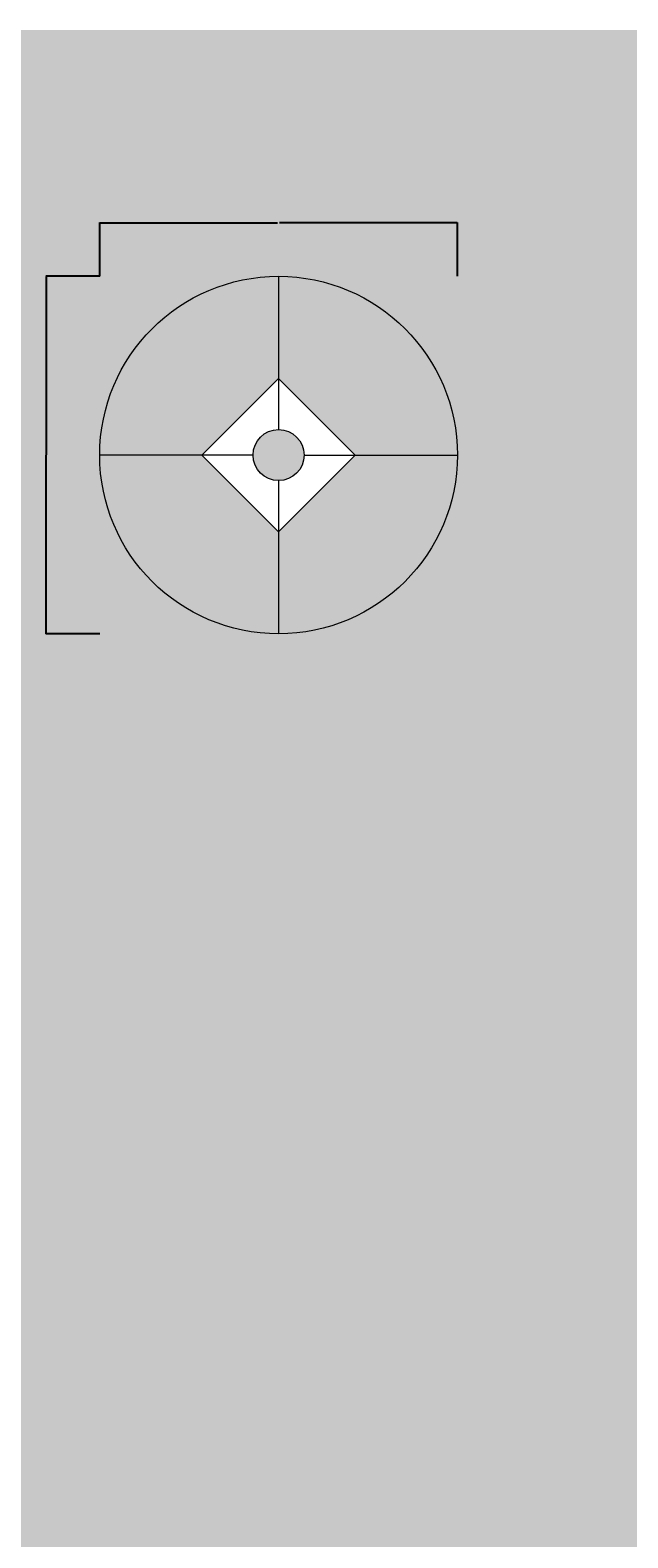
# Model space of a CAD drawing. Units: millimetres. Extents: x -229 to 16545, y -10488 to 4272.
# Tile 19 of 29: x 10978 to 11572, y -2708 to -1208. Entities that reach past the tile are written whole.
import ezdxf

# ---------------------------------------------------------------- set-up
doc = ezdxf.new("R2010")
doc.units = ezdxf.units.MM
for name, color, linetype, lineweight in [('A-ANNO-DIMS', 2, 'Continuous', 18), ('A-FURN', 8, 'Continuous', 18), ('A-FURN-PATT', 252, 'Continuous', 13)]:
    doc.layers.add(name, color=color, linetype=linetype, lineweight=lineweight)
doc.layers.add('A-FLOR-PATT', color=254, linetype='Continuous', lineweight=13, true_color=0xfeeab9)
doc.styles.get("Standard").update_dxf_attribs({"font": 'arial.ttf'})
doc.dimstyles.get("Standard").update_dxf_attribs({"dimtxt": 0.18, "dimasz": 0.18, "dimexe": 0.18, "dimexo": 0.0625, "dimgap": 0.09, "dimtad": 0, "dimtih": 1, "dimtoh": 1, "dimdec": 4, "dimzin": 0, "dimdsep": 46, "dimtxsty": 'Standard', "dimcen": 0.09, "dimadec": 0, "dimazin": 0, "dimtfac": 1, "dimtdec": 4, "dimtofl": 0, "dimtmove": 0, "dimatfit": 3, "dimfxl": 1, "dimtolj": 1, "dimtzin": 0, "dimarcsym": 0})

# ---------------------------------------------------------------- blocks, each defined once
blk = doc.blocks.new('Lamp - Table')
for p, q in [((0, 7), (0, 1)), ((0, 3), (-3, 0)), ((3, 0), (0, 3)), ((-1, 0), (-7, 0)), ((-3, 0), (0, -3)), ((0, -3), (3, 0)), ((1, 0), (7, 0)), ((0, -1), (0, -7))]:
    blk.add_line(p, q)
for radius in [7, 1]:
    blk.add_circle((0, 0), radius)
blk = doc.blocks.new('*D27')
at = {"layer": 'A-ANNO-DIMS', "color": 0, "lineweight": -2, "transparency": 16777216}
for p, q in [((11047.2, -1453.1), (11047.2, -1399.6)), ((11047.4, -1399.8), (11224, -1399.8)), ((11402.6, -1399.8), (11226, -1399.8)), ((11402.8, -1453.1), (11402.8, -1399.6))]:
    blk.add_line(p, q, dxfattribs=at)
at = {"layer": 'A-ANNO-DIMS', "color": 0, "transparency": 16777216}
for points in [[(11047.4, -1399.8), (11047.4, -1399.8), (11047.2, -1399.8)], [(11402.6, -1399.8), (11402.6, -1399.8), (11402.8, -1399.8)]]:
    blk.add_solid(points, dxfattribs=at)
at = {"layer": 'Defpoints', "color": 0, "transparency": 16777216}
for p in [(11402.8, -1399.8), (11047.2, -1453.1), (11402.8, -1453.1)]:
    blk.add_point(p, dxfattribs=at)
at = {"layer": 'A-ANNO-DIMS', "color": 0, "transparency": 16777216, "insert": (11225, -1399.8), "char_height": 0.18, "attachment_point": 5}
blk.add_mtext('\\A1;LAMP 356 TYP.', dxfattribs=at)
blk = doc.blocks.new('*D28')
at = {"layer": 'A-ANNO-DIMS', "color": 0, "lineweight": -2, "transparency": 16777216}
for p, q in [((11047.2, -1453.1), (10993.7, -1453.1)), ((10993.9, -1453.3), (10993.9, -1630.8)), ((10993.9, -1808.6), (10993.9, -1631.1)), ((11047.2, -1808.7), (10993.7, -1808.7))]:
    blk.add_line(p, q, dxfattribs=at)
at = {"layer": 'A-ANNO-DIMS', "color": 0, "transparency": 16777216}
for points in [[(10993.8, -1453.3), (10993.9, -1453.3), (10993.9, -1453.1)], [(10993.8, -1808.6), (10993.9, -1808.6), (10993.9, -1808.7)]]:
    blk.add_solid(points, dxfattribs=at)
at = {"layer": 'Defpoints', "color": 0, "transparency": 16777216}
for p in [(10993.9, -1453.1), (11047.2, -1453.1), (11047.2, -1808.7)]:
    blk.add_point(p, dxfattribs=at)
at = {"layer": 'A-ANNO-DIMS', "color": 0, "transparency": 16777216, "insert": (10993.9, -1630.9), "char_height": 0.18, "attachment_point": 5}
blk.add_mtext('\\A1;356 TYP.', dxfattribs=at)

msp = doc.modelspace()

# ---------------------------------------------------------------- hatches: boundary and pattern name
at = {"layer": 'A-FLOR-PATT', "transparency": 33554592}
h = msp.add_hatch(color=256, dxfattribs=at)
h.dxf.hatch_style = 1
h.paths.add_polyline_path([(7975.933, -5325.772), (7943.121, -5325.772), (7943.121, -4576.49, 0.40145271), (7225.933, -5325.772, 0.40145271), (6508.746, -4576.49), (6508.746, -5325.772), (6475.933, -5325.772), (6475.933, -5438.272), (5975.933, -5438.272), (5975.933, -7267.724), (5975.933, -7438.272), (6478.619, -7438.272), (6463.448, -7355.919), (6464.88, -7356.837), (6463.849, -7358.097), (6478.619, -7438.272), (6610.327, -7438.272), (6632.656, -7409.564), (6632.525, -7406.967), (6634.208, -7407.569), (6619.273, -7426.77), (6654.466, -7438.272), (7610.517, -7438.272), (7607.41, -7421.409), (7608.842, -7422.327), (7607.812, -7423.587), (7610.517, -7438.272), (7975.933, -7438.272)])
h.paths.add_polyline_path([(13785.933, -1208.272), (9555.933, -1208.272), (9555.933, -961.785), (9705.933, -961.785), (9705.933, -918.035), (10704.976, -918.035, 0.40145271), (9705.933, 38.215), (9555.933, 38.215), (9555.933, 2021.728), (5975.933, 2021.728), (5975.933, 755.492), (5745.933, 755.492), (5745.933, 1427.266), (2918.813, 1427.266), (2918.813, -492.942), (5013.319, -492.942), (5013.319, -978.272), (5745.933, -978.272), (5745.933, -397.513), (5975.933, -397.513), (5975.933, -1208.272), (4560.933, -1208.272), (4560.933, -1265.772), (4448.433, -1265.772), (4448.433, -1298.585), (4445.933, -1298.585), (3699.151, -1298.585, 0.40145271), (4448.433, -2015.772), (4560.933, -2015.772), (4560.933, -2384.177), (5745.933, -2384.177), (5799.402, -2384.177), (5799.402, -4518.272), (5975.933, -4518.272), (5975.933, -5208.272), (6475.933, -5208.272), (6475.933, -4575.772), (6508.746, -4575.772), (6508.746, -4576.49, -0.35647263), (7216.672, -5208.272), (7235.194, -5208.272, -0.35647263), (7943.121, -4576.49), (7943.121, -4575.772), (7975.933, -4575.772), (7975.933, -5208.272), (11176.247, -5208.272), (11159.44, -5191.465), (10520.768, -5191.465), (10520.768, -4888.936), (10571.19, -4888.936), (10571.19, -4872.129), (10772.876, -4872.129), (10772.876, -4888.936), (10789.683, -4888.936), (10789.683, -4872.129), (10991.368, -4872.129), (10991.368, -4888.936), (11041.79, -4888.936), (11041.79, -4872.129), (11058.597, -4872.129, -0.09090909), (11428.354, -4872.129), (11445.162, -4872.129), (11445.162, -4888.936), (11529.197, -4888.936), (11529.197, -5191.465), (11327.512, -5191.465), (11310.704, -5208.272), (13785.933, -5208.272)])
h.paths.add_polyline_path([(11047.216, -1630.944, -1), (11402.816, -1630.944, -1)], flags=16)
h.paths.add_polyline_path([(11148.816, -1630.944), (11225.016, -1554.744), (11301.216, -1630.944), (11225.016, -1707.144)], flags=0)
h.paths.add_polyline_path([(11199.616, -1630.944, -1), (11250.416, -1630.944, -1)], flags=0)
h.paths.add_polyline_path([(11588.751, -2096.259), (11588.751, -1543.254, -0.26666697), (12864.918, -1543.254), (12864.918, -2096.259), (12737.302, -2096.259), (12737.302, -2063.121), (11716.368, -2063.121), (11716.368, -2096.259)], flags=16)
h.paths.add_polyline_path([(12012.696, -2489.42), (12600.997, -2489.42), (12600.997, -3666.022), (12012.696, -3666.022)], flags=16)
h.paths.add_polyline_path([(12176.41, -3599.403), (12174.938, -3609.076), (12173.789, -3618.819), (12173.09, -3628.559), (12172.973, -3638.221), (12173.89, -3652.852), (12175.008, -3657.025), (12172.909, -3643.473), (12173.142, -3624.297), (12175.386, -3605.273)], flags=0)
h.paths.add_polyline_path([(8026.289, -286.944), (7737.703, -287.19), (7734.87, -269.156), (8029.092, -268.905)], flags=16)
h.paths.add_polyline_path([(7733.453, -260.139), (7710.784, -115.865), (7557.191, -115.996), (7556.999, 109.744), (7412.687, 132.166), (7412.433, 429.206), (7556.707, 451.876), (7556.568, 614.769), (7412.256, 637.19), (7412.003, 934.231), (7556.276, 956.9), (7556.084, 1182.639), (7709.677, 1182.77), (7732.099, 1327.082), (8029.14, 1327.335), (8051.808, 1183.062), (8205.401, 1183.192), (8205.594, 957.454), (8349.906, 935.031), (8350.159, 637.99), (8205.885, 615.322), (8206.024, 452.43), (8350.336, 430.006), (8350.59, 132.965), (8206.316, 110.298), (8206.509, -115.442), (8052.916, -115.573), (8030.493, -259.885)], flags=16)
h.paths.add_polyline_path([(12261.416, -3475.554), (12262.632, -3486.776), (12264.032, -3497.007), (12265.554, -3506.365), (12267.136, -3514.968), (12268.719, -3522.935), (12271.304, -3535.59), (12273.606, -3548.078), (12275.271, -3561.064), (12275.93, -3574.938), (12275.325, -3590.3), (12273.425, -3607.964), (12270.795, -3625.658), (12268.066, -3641.063), (12266.318, -3649.679), (12265.456, -3653.626), (12263.984, -3659.846), (12264.032, -3659.566), (12264.342, -3658.241), (12264.807, -3656.37), (12265.456, -3653.626), (12266.318, -3649.679), (12267.409, -3644.302), (12268.668, -3637.664), (12270.019, -3630.037), (12271.384, -3621.695), (12272.69, -3612.908), (12273.857, -3603.948), (12274.81, -3595.088), (12275.47, -3586.601), (12275.782, -3578.689), (12275.757, -3571.292), (12275.423, -3564.275), (12274.816, -3557.512), (12273.964, -3550.872), (12272.896, -3544.224), (12271.645, -3537.439), (12270.24, -3530.385), (12267.543, -3517.181), (12264.612, -3501.247), (12261.849, -3481.059)], flags=0)
h.paths.add_polyline_path([(12332.136, -3408.03), (12333.483, -3416.79), (12335.077, -3424.54), (12336.915, -3431.355), (12338.991, -3437.32), (12341.266, -3442.55), (12343.694, -3447.166), (12346.229, -3451.292), (12348.826, -3455.051), (12351.438, -3458.563), (12357.476, -3466.491), (12363.61, -3476.575), (12368.309, -3489.762), (12369.929, -3503.427), (12369.842, -3516.511), (12368.43, -3530.867), (12365.816, -3545.835), (12362.382, -3559.786), (12360.968, -3564.487), (12363.063, -3557.021), (12364.898, -3549.566), (12366.473, -3542.077), (12367.773, -3534.631), (12368.781, -3527.301), (12369.483, -3520.162), (12369.863, -3513.291), (12369.906, -3506.759), (12369.599, -3500.643), (12368.93, -3494.999), (12367.924, -3489.796), (12366.61, -3484.994), (12365.024, -3480.542), (12363.19, -3476.399), (12361.141, -3472.516), (12358.909, -3468.847), (12356.525, -3465.347), (12354.02, -3461.954), (12351.438, -3458.563), (12345.462, -3450.529), (12339.923, -3439.996), (12335.85, -3428.296), (12332.68, -3412.888)], flags=0)
h.paths.add_polyline_path([(12385.287, -3334.612), (12384.977, -3342.409), (12385.02, -3349.196), (12385.4, -3355.066), (12386.104, -3360.105), (12387.112, -3364.41), (12388.412, -3368.071), (12389.987, -3371.181), (12391.823, -3373.832), (12393.919, -3376.097), (12396.337, -3377.978), (12399.153, -3379.462), (12402.445, -3380.531), (12406.289, -3381.172), (12410.758, -3381.371), (12415.935, -3381.106), (12421.893, -3380.368), (12428.658, -3379.159), (12436.069, -3377.55), (12443.907, -3375.635), (12451.961, -3373.505), (12460.015, -3371.254), (12467.853, -3368.971), (12475.263, -3366.749), (12482.029, -3364.68), (12491.877, -3361.657), (12497.701, -3360.107), (12501.639, -3359.288), (12510.135, -3358.326), (12519.662, -3365.412), (12524.243, -3378.911), (12523.764, -3390.7), (12520.746, -3401.577), (12514.248, -3415.634), (12511.518, -3420.418), (12515.856, -3412.154), (12519.153, -3405.024), (12521.516, -3398.804), (12523.049, -3393.276), (12523.865, -3388.212), (12524.059, -3383.441), (12523.7, -3378.958), (12522.853, -3374.815), (12521.576, -3371.054), (12519.931, -3367.722), (12517.982, -3364.865), (12515.786, -3362.529), (12513.405, -3360.758), (12510.877, -3359.588), (12508.136, -3358.982), (12505.086, -3358.897), (12501.639, -3359.288), (12497.701, -3360.107), (12493.183, -3361.309), (12487.988, -3362.851), (12476.403, -3366.408), (12463.335, -3370.326), (12447.372, -3374.788), (12431.759, -3378.604), (12418.504, -3380.974), (12405.811, -3381.624), (12394.725, -3378.025), (12388.039, -3368.367), (12385.583, -3357.877), (12384.826, -3346.204), (12385.428, -3331.059), (12385.953, -3325.719)], flags=0)
h.paths.add_polyline_path([(7880.016, 1173.969), (7880.373, 1175.495), (7880.433, 1175.851), (7879.484, 1171.818)], flags=0)
h.paths.add_polyline_path([(7802.33, 874.962), (7800.771, 885.032), (7798.932, 893.941), (7796.811, 901.774), (7794.419, 908.63), (7791.798, 914.639), (7789.002, 919.945), (7786.083, 924.686), (7783.093, 929.005), (7780.087, 933.043), (7774.996, 939.717), (7768.406, 949.37), (7762.174, 963.427), (7759.342, 978.002), (7758.629, 991.888), (7759.492, 1007.928), (7761.801, 1025.496), (7765.392, 1044.035), (7766.625, 1049.048), (7764.522, 1039.543), (7762.719, 1030.232), (7761.232, 1021.168), (7760.08, 1012.405), (7759.28, 1003.994), (7758.849, 995.988), (7758.806, 988.44), (7759.167, 981.404), (7759.942, 974.914), (7761.104, 968.936), (7762.617, 963.414), (7764.448, 958.299), (7766.559, 953.535), (7768.918, 949.073), (7771.487, 944.856), (7774.232, 940.835), (7777.115, 936.938), (7782.377, 930.041), (7787.845, 922.139), (7793.348, 911.698), (7798.042, 898.247), (7801.702, 880.527)], flags=0)
h.paths.add_polyline_path([(12519.068, -3228.534), (12519.615, -3236.235), (12520.529, -3242.343), (12521.78, -3247.103), (12523.337, -3250.758), (12525.171, -3253.556), (12527.248, -3255.709), (12529.522, -3257.296), (12531.95, -3258.361), (12534.486, -3258.949), (12537.082, -3259.11), (12539.694, -3258.888), (12542.277, -3258.329), (12544.781, -3257.478), (12547.173, -3256.388), (12549.46, -3255.129), (12550.455, -3254.517), (12555.825, -3251.109), (12557.835, -3249.942), (12565.181, -3246.404), (12574.565, -3253.032), (12576.931, -3265.022), (12576.627, -3277.425), (12575.416, -3290.819), (12574.851, -3295.392), (12575.708, -3287.593), (12576.322, -3280.806), (12576.688, -3274.939), (12576.812, -3269.899), (12576.688, -3265.593), (12576.322, -3261.932), (12575.708, -3258.822), (12574.851, -3256.172), (12573.753, -3253.905), (12572.439, -3252.005), (12570.943, -3250.474), (12569.293, -3249.309), (12567.523, -3248.513), (12565.658, -3248.083), (12563.732, -3248.022), (12561.777, -3248.328), (12559.814, -3248.989), (12557.835, -3249.942), (12555.825, -3251.109), (12553.77, -3252.413), (12551.652, -3253.78), (12549.46, -3255.129), (12543.167, -3258.594), (12532.661, -3259.485), (12524.685, -3253.923), (12520.949, -3245.152), (12519.138, -3233.042)], flags=0)
h.paths.add_polyline_path([(7741.293, 790.501), (7741.641, 799.467), (7741.584, 807.269), (7741.141, 814.015), (7740.329, 819.809), (7739.165, 824.757), (7737.667, 828.966), (7735.853, 832.541), (7733.74, 835.586), (7731.348, 838.188), (7728.71, 840.348), (7725.861, 842.052), (7722.836, 843.28), (7719.671, 844.015), (7716.4, 844.237), (7713.06, 843.932), (7709.684, 843.081), (7706.304, 841.686), (7702.923, 839.834), (7699.543, 837.629), (7696.164, 835.178), (7692.784, 832.585), (7684.718, 826.315), (7675.609, 820.63), (7664.001, 817.274), (7654.105, 821.884), (7647.171, 832.02), (7644.191, 846.522), (7646.321, 860.288), (7647.49, 864.223), (7645.946, 857.865), (7645.046, 852.044), (7644.827, 846.557), (7645.243, 841.404), (7646.221, 836.642), (7647.693, 832.318), (7649.587, 828.489), (7651.832, 825.206), (7654.359, 822.523), (7657.097, 820.49), (7659.984, 819.145), (7662.993, 818.452), (7666.108, 818.357), (7669.311, 818.809), (7672.583, 819.755), (7675.908, 821.139), (7679.268, 822.913), (7682.645, 825.021), (7686.025, 827.401), (7689.404, 829.958), (7692.784, 832.585), (7700.505, 838.509), (7709.871, 843.64), (7721.436, 844.698), (7733.277, 837.617), (7739.571, 825.214), (7741.557, 811.049), (7741.669, 795.575)], flags=0)
h.paths.add_polyline_path([(8377.641, 137.216), (8359.607, 134.382), (8359.356, 428.605), (8377.395, 425.802)], flags=16)
h.paths.add_polyline_path([(7650.715, 668.465), (7650.08, 677.319), (7649.023, 684.34), (7647.579, 689.811), (7645.785, 694.012), (7643.675, 697.228), (7641.286, 699.7), (7638.669, 701.521), (7635.876, 702.744), (7632.96, 703.419), (7629.974, 703.601), (7626.971, 703.344), (7624.004, 702.697), (7621.125, 701.717), (7618.375, 700.462), (7615.749, 699.013), (7614.561, 698.279), (7608.435, 694.382), (7606.125, 693.04), (7598.981, 689.594), (7589.669, 693.773), (7585.26, 702.856), (7584.221, 713.11), (7584.49, 724.584), (7585.863, 739.937), (7586.518, 745.277), (7585.539, 736.31), (7584.841, 728.507), (7584.424, 721.761), (7584.288, 715.966), (7584.433, 711.016), (7584.86, 706.807), (7585.567, 703.231), (7586.556, 700.186), (7587.821, 697.58), (7589.332, 695.397), (7591.053, 693.637), (7592.951, 692.3), (7594.989, 691.385), (7597.132, 690.895), (7599.346, 690.826), (7601.594, 691.18), (7603.851, 691.943), (7606.125, 693.04), (7608.435, 694.382), (7610.797, 695.885), (7613.229, 697.458), (7620.475, 701.929), (7632.001, 704.44), (7643.476, 699.417), (7648.536, 687.571), (7650.63, 673.661)], flags=0)
h.paths.add_polyline_path([(7385.628, 136.37), (7385.382, 424.956), (7403.416, 427.789), (7403.667, 133.567)], flags=16)
h.paths.add_polyline_path([(12993.884, -2257.186), (12959.588, -2257.186), (12959.588, -2125.099), (13531.966, -2125.099, -0.19047621), (13531.966, -3974.321), (12959.588, -3974.321), (12959.588, -3842.233), (12993.884, -3842.233)], flags=16)
h.paths.add_polyline_path([(13413.486, -3313.884), (13413.486, -2785.535), (13562.885, -2785.535, -0.04962821), (13562.885, -3313.884)], flags=0)
h.paths.add_polyline_path([(8377.21, 642.241), (8359.176, 639.407), (8358.925, 933.629), (8376.964, 930.826)], flags=16)
h.paths.add_polyline_path([(13086.058, -1864.83), (13086.058, -1449.84), (13501.048, -1449.84), (13501.048, -1864.83)], flags=16)
h.paths.add_polyline_path([(13305.814, -1862.197), (13302.103, -1859.624), (13298.088, -1857.068), (13293.799, -1854.536), (13289.262, -1852.031), (13284.504, -1849.559), (13279.554, -1847.125), (13274.439, -1844.735), (13269.17, -1842.389), (13263.701, -1840.081), (13257.97, -1837.797), (13251.914, -1835.525), (13245.472, -1833.252), (13238.582, -1830.968), (13231.18, -1828.66), (13223.206, -1826.315), (13209.182, -1822.458), (13204.584, -1821.48), (13217.962, -1824.773), (13235.072, -1829.804), (13248.777, -1834.349), (13260.829, -1838.869), (13274.479, -1844.63), (13289.675, -1852.101), (13302.553, -1859.704)], flags=0)
h.paths.add_polyline_path([(13428.104, -1820.994), (13419.007, -1818.141), (13409.95, -1815.4), (13400.766, -1812.747), (13391.271, -1810.151), (13376.087, -1806.251), (13370.618, -1805.019), (13386.304, -1808.794), (13405.087, -1813.928), (13423.014, -1819.354)], flags=0)
h.paths.add_polyline_path([(7385.197, 641.395), (7384.951, 929.98), (7402.986, 932.814), (7403.236, 638.592)], flags=16)
h.paths.add_polyline_path([(13262.537, -1725.526), (13253.246, -1724.74), (13244.516, -1724.117), (13235.94, -1723.625), (13223.267, -1723.062), (13217.598, -1722.912), (13231.966, -1723.397), (13248.733, -1724.359), (13266.899, -1725.895), (13272.802, -1726.502)], flags=0)
h.paths.add_polyline_path([(13191.893, -1641.137), (13208.675, -1640.506), (13214.057, -1640.258), (13197.763, -1640.936)], flags=0)
h.paths.add_polyline_path([(13097.524, -1608.457), (13114.284, -1609.031), (13120.126, -1609.105), (13103.045, -1608.71)], flags=0)
h.paths.add_polyline_path([(13465.328, -1521.577), (13473.906, -1517.015), (13481.761, -1511.636), (13492.562, -1502.076), (13495.327, -1497.933), (13485.818, -1508.858), (13470.208, -1519.547)], flags=0)
h.paths.add_polyline_path([(13175.015, -1500.891), (13184.046, -1501.807), (13192.721, -1502.52), (13201.114, -1503.034), (13209.273, -1503.351), (13217.244, -1503.476), (13225.078, -1503.41), (13232.821, -1503.16), (13240.524, -1502.728), (13248.233, -1502.117), (13255.993, -1501.322), (13263.825, -1500.293), (13271.746, -1498.974), (13279.775, -1497.305), (13287.928, -1495.229), (13296.222, -1492.688), (13304.675, -1489.622), (13313.304, -1485.975), (13322.089, -1481.727), (13330.859, -1477.028), (13339.408, -1472.063), (13347.526, -1467.02), (13355.006, -1462.087), (13364.86, -1455.202), (13367.224, -1453.299), (13358.544, -1459.754), (13343.348, -1469.775), (13326.143, -1479.767), (13309.023, -1488.045), (13292.249, -1494.129), (13276.009, -1498.264), (13260.299, -1500.88), (13244.401, -1502.51), (13228.945, -1503.378), (13213.316, -1503.508), (13197.047, -1502.876), (13180.088, -1501.481)], flags=0)
h.paths.add_polyline_path([(7733.501, 1336.101), (7736.303, 1354.14), (8024.889, 1354.386), (8027.723, 1336.352)], flags=16)
at = {"layer": 'A-FURN-PATT'}
h = msp.add_hatch(color=256, dxfattribs=at)
h.dxf.hatch_style = 1
h.paths.add_polyline_path([(13549.668, 1603.014, 0.41421356), (13371.868, 1425.214), (13473.468, 1425.214), (13549.668, 1501.414)])
h.paths.add_polyline_path([(13549.668, 1603.014), (13549.668, 1501.414), (13625.868, 1425.214), (13727.468, 1425.214, 0.41421356)])
h.paths.add_polyline_path([(13727.468, 1425.214), (13625.868, 1425.214), (13549.668, 1349.014), (13549.668, 1247.414, 0.41421356)])
h.paths.add_polyline_path([(13473.468, 1425.214), (13371.868, 1425.214, 0.41421356), (13549.668, 1247.414), (13549.668, 1349.014)])
h.paths.add_polyline_path([(13524.268, 1425.214, 1), (13575.068, 1425.214, 1)])
h.paths.add_polyline_path([(11148.816, -1630.944), (11047.216, -1630.944, 0.41421356), (11225.016, -1808.744), (11225.016, -1707.144)])
h.paths.add_polyline_path([(11402.816, -1630.944), (11301.216, -1630.944), (11225.016, -1707.144), (11225.016, -1808.744, 0.41421356)])
h.paths.add_polyline_path([(11225.016, -1453.144, 0.41421356), (11047.216, -1630.944), (11148.816, -1630.944), (11225.016, -1554.744)])
h.paths.add_polyline_path([(11225.016, -1453.144), (11225.016, -1554.744), (11301.216, -1630.944), (11402.816, -1630.944, 0.41421356)])
h.paths.add_polyline_path([(11199.616, -1630.944, 1), (11250.416, -1630.944, 1)])

# ---------------------------------------------------------------- block references
at = {"layer": 'A-FURN', "xscale": 25.4, "yscale": 25.4, "zscale": 25.4}
msp.add_blockref('Lamp - Table', (11225.016, -1630.944), dxfattribs=at)

# ---------------------------------------------------------------- dimensions: what is measured, and where the dimension line sits
at = {"layer": 'A-ANNO-DIMS'}
dim = msp.add_linear_dim(base=(11402.816, -1399.804), p1=(11047.216, -1453.144), p2=(11402.816, -1453.144), text='LAMP <> TYP.', dimstyle='Standard', override={"dimdec": 0, "dimlfac": 1, "dimrnd": 0, "dimzin": 0, "dimdsep": 46, "dimlunit": 2}, dxfattribs=at)
dim.commit()
dim.dimension.update_dxf_attribs({"geometry": '*D27', "text_midpoint": (11225.016, -1399.804)})
dim = msp.add_linear_dim(base=(10993.876, -1453.144), p1=(11047.216, -1808.744), p2=(11047.216, -1453.144), angle=90, text='<> TYP.', dimstyle='Standard', override={"dimdec": 0, "dimlfac": 1, "dimrnd": 0, "dimzin": 0, "dimdsep": 46, "dimlunit": 2}, dxfattribs=at)
dim.commit()
dim.dimension.update_dxf_attribs({"geometry": '*D28', "text_midpoint": (10993.876, -1630.944)})

doc.saveas('drawing.dxf')
